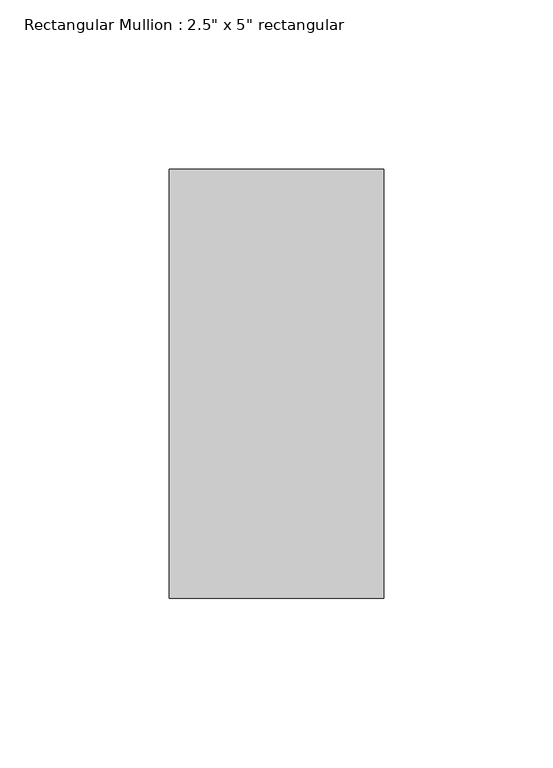
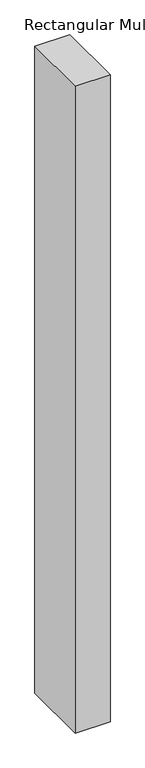
"""IFC4 building model written with IfcOpenShell, lengths in millimetres: member geometry."""

from ifc_helpers import new_model, si_unit, frame, origin, place, context, project, spatial, polyline, outline, extrude, source, transform, mapped, element, save


def member_71eb4692(model_context):
    return source(origin(), model_context, "Body", "SweptSolid", [
        extrude(outline(polyline([(0.0, 63.5), (0.0, -63.5), (-63.5, -63.5), (-63.5, 63.5), (0.0, 63.5)])), frame((0.0, 0.0, -1244.6), z_axis=(0.0, 0.0, 1.0), x_axis=(1.0, 0.0, 0.0)), (0.0, 0.0, 1.0), 1244.6),
    ])


if __name__ == "__main__":
    model = new_model("IFC4")
    model_context = context("Model", 3, world=origin())
    ifc_project = project(units=[si_unit("LENGTHUNIT", "METRE", prefix="MILLI")], contexts=[model_context])
    site = spatial("IfcSite", under=ifc_project)
    building = spatial("IfcBuilding", under=site)
    placement = place(None, origin())
    member_shape = member_71eb4692(model_context)
    element("IfcMember", 1, ObjectType="Rectangular Mullion : 2.5\" x 5\" rectangular", at=placement, inside=building, context=model_context, shape_type="MappedRepresentation", body=[
        mapped(member_shape, transform((0.0, 0.0, 0.0), x_axis=(1.0, 0.0, 0.0), y_axis=(0.0, 1.0, 0.0), z_axis=(0.0, 0.0, 1.0))),
    ])
    save(model, "model.ifc")

# Revit data of these elements
# Type "Rectangular Mullion : 2.5\" x 5\" rectangular"
#   built-in parameter 1007304 = 0.416667 (stored number, unit not read)
#   built-in parameter 1007301 = 0.104167 (stored number, unit not read)
#   built-in parameter 1007300 = 0.104167 (stored number, unit not read)
